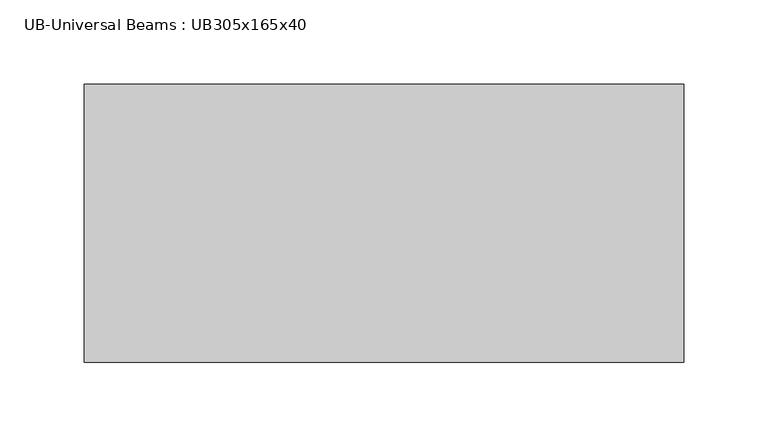
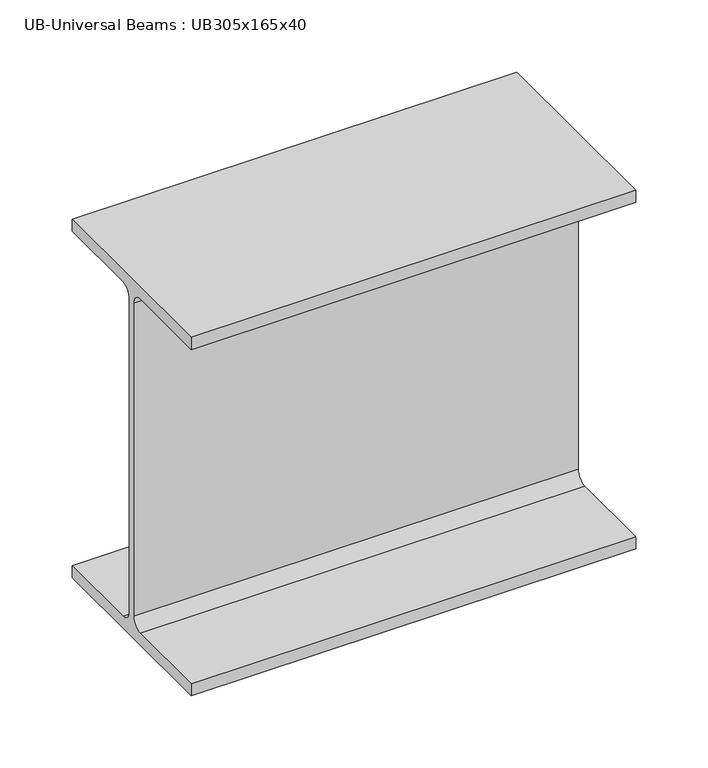
"""IFC4 building model written with IfcOpenShell, lengths in millimetres: beam geometry, UB-Universal Beams : UB305x165x40."""

from ifc_helpers import new_model, si_unit, point, frame, frame_2d, origin, place, context, project, spatial, polyline, circle_curve, trimmed, segment, composite_curve, outline, extrude, source, transform, mapped, element, save


def ub_universal_beams_ub305x165x40_fca44d3c(model_context):
    return source(origin(), model_context, "Body", "SweptSolid", [
        extrude(outline(composite_curve([segment(polyline([(-82.5, -141.5), (-11.9, -141.5)]), True, "CONTINUOUS"), segment(trimmed(circle_curve(frame_2d((-11.9, -132.6)), 8.9), [point((-11.9, -141.5))], [point((-3.0, -132.6))], True, "CARTESIAN"), True, "CONTINUOUS"), segment(polyline([(-3.0, -132.6), (-3.0, 132.6)]), True, "CONTINUOUS"), segment(trimmed(circle_curve(frame_2d((-11.9, 132.6)), 8.9), [point((-3.0, 132.6))], [point((-11.9, 141.5))], True, "CARTESIAN"), True, "CONTINUOUS"), segment(polyline([(-11.9, 141.5), (-82.5, 141.5), (-82.5, 151.7), (82.5, 151.7), (82.5, 141.5), (11.9, 141.5)]), True, "CONTINUOUS"), segment(trimmed(circle_curve(frame_2d((11.9, 132.6)), 8.9), [point((11.9, 141.5))], [point((3.0, 132.6))], True, "CARTESIAN"), True, "CONTINUOUS"), segment(polyline([(3.0, 132.6), (3.0, -132.6)]), True, "CONTINUOUS"), segment(trimmed(circle_curve(frame_2d((11.9, -132.6)), 8.9), [point((3.0, -132.6))], [point((11.9, -141.5))], True, "CARTESIAN"), True, "CONTINUOUS"), segment(polyline([(11.9, -141.5), (82.5, -141.5), (82.5, -151.7), (-82.5, -151.7), (-82.5, -141.5)]), True, "CONTINUOUS")], self_intersect=False)), frame((309.65, 0.0, 0.0), z_axis=(1.0, 0.0, 0.0), x_axis=(0.0, 1.0, 0.0)), (0.0, 0.0, 1.0), 355.9),
    ])


if __name__ == "__main__":
    model = new_model("IFC4")
    model_context = context("Model", 3, world=origin())
    ifc_project = project(units=[si_unit("LENGTHUNIT", "METRE", prefix="MILLI")], contexts=[model_context])
    site = spatial("IfcSite", under=ifc_project)
    building = spatial("IfcBuilding", under=site)
    placement = place(None, origin())
    ub_universal_beams_ub305x165x40_shape = ub_universal_beams_ub305x165x40_fca44d3c(model_context)
    element("IfcBeam", 1, ObjectType="UB-Universal Beams : UB305x165x40", at=placement, inside=building, context=model_context, shape_type="MappedRepresentation", body=[
        mapped(ub_universal_beams_ub305x165x40_shape, transform((0.0, 0.0, 0.0), x_axis=(1.0, 0.0, 0.0), y_axis=(0.0, 1.0, 0.0), z_axis=(0.0, 0.0, 1.0))),
    ])
    save(model, "model.ifc")

# Revit data of these elements
# Type "UB-Universal Beams : UB305x165x40"
#   Section Name Key = "UB305X165X40"
#   Width = 16.5 cm
#   Web Thickness = 0.6 cm
#   Web Fillet = 0.89 cm
#   Warping Constant = 164000.0 cm⁶
#   Torsional Moment of Inertia = 14.70 cm⁴
#   Section Area = 51.3 cm²
#   Plastic Modulus weak axis = 142.0 cm³
#   Plastic Modulus strong axis = 623.0 cm³
#   Nominal Weight = 40.2999 kgf/m
#   Moment of Inertia weak axis = 764.00 cm⁴
#   Moment of Inertia strong axis = 8503.00 cm⁴
#   Height = 30.34 cm
#   Flange Thickness = 1.02 cm
#   Elastic Modulus weak axis = 92.6 cm³
#   Elastic Modulus strong axis = 560.0 cm³
#   Centroid Vertical = 15.17 cm
#   Centroid Horizontal = 8.25 cm
#   Bolt Spacing = 9.0 cm
#   Length [instance default] = 1500 mm
#   Structural Material [instance default] = Metal - Steel 43-275
#   Type Comments = ""
#   Assembly Code = ""
# Element 1 (IfcBeam, "UB-Universal Beams : UB305x165x40")
#   Materials on its faces: "Metal - Steel 43-275"
# Materials
#   "Metal - Steel 43-275": class "Metal", colour RGB 247 247 247, transparency 0, Cost = 0
